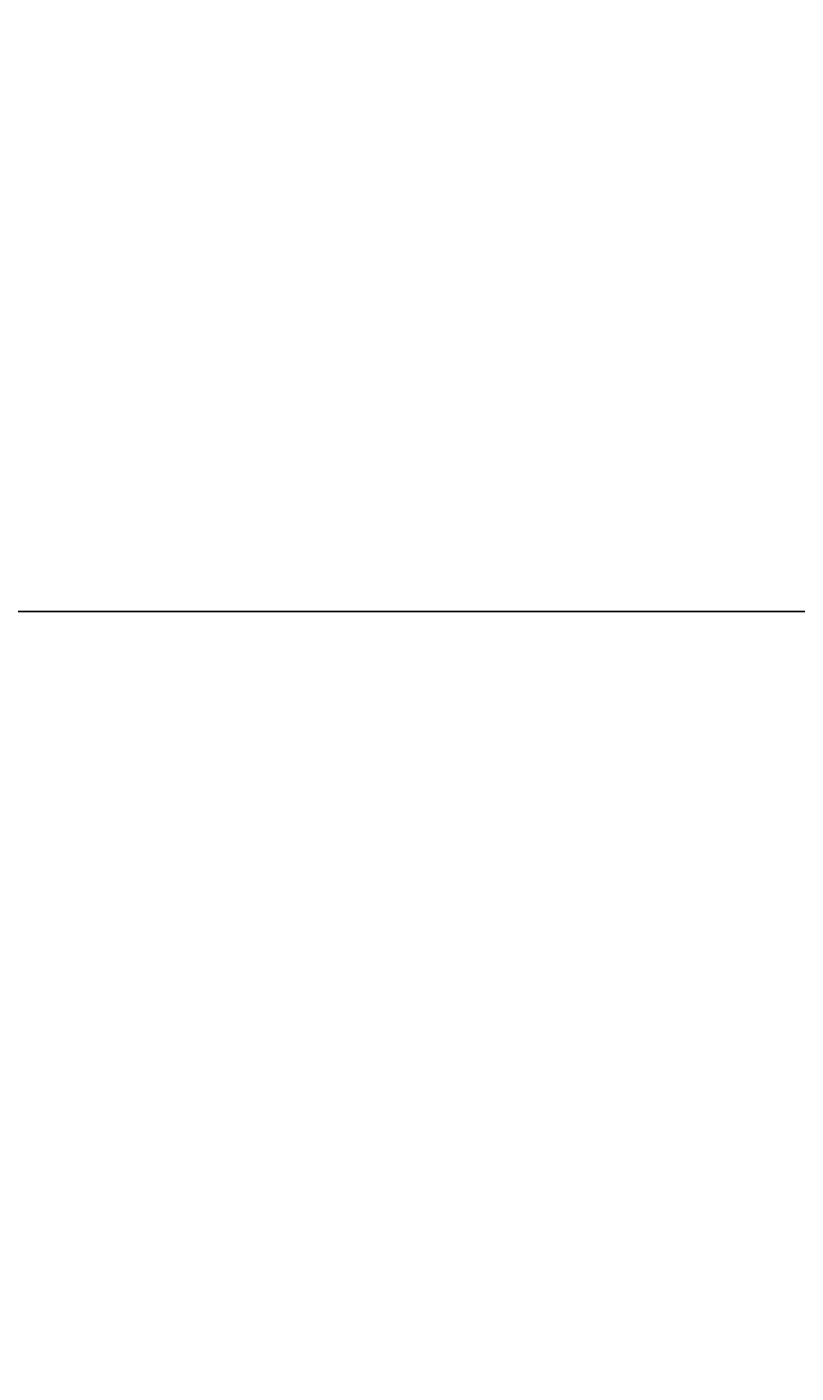
# Model space of a CAD drawing. Units: inches. Extents: x -301 to 715, y -607 to 364.
# Tile 38 of 141: x 101 to 121, y -405 to -370. Entities that reach past the tile are written whole.
import ezdxf

# ---------------------------------------------------------------- set-up
doc = ezdxf.new("R2010")
doc.units = ezdxf.units.IN
doc.header["$MEASUREMENT"] = 0
doc.layers.add('A-ANNO-DIMS', color=2, linetype='Continuous', lineweight=18)
doc.styles.get("Standard").update_dxf_attribs({"font": 'arial.ttf'})
doc.dimstyles.get("Standard").update_dxf_attribs({"dimtxt": 0.18, "dimasz": 0.18, "dimexe": 0.18, "dimexo": 0.0625, "dimgap": 0.09, "dimtad": 0, "dimtih": 1, "dimtoh": 1, "dimdec": 1, "dimzin": 0, "dimdsep": 46, "dimlunit": 4, "dimtxsty": 'Standard', "dimcen": 0.09, "dimclrd": 3, "dimclre": 4, "dimclrt": 6, "dimadec": 0, "dimazin": 0, "dimtfac": 1, "dimtdec": 1, "dimtofl": 0, "dimtmove": 0, "dimatfit": 3, "dimfxl": 1, "dimtfill": 2, "dimtfillclr": 51, "dimtolj": 1, "dimtzin": 0, "dimarcsym": 0})

# ---------------------------------------------------------------- blocks, each defined once
blk = doc.blocks.new('*D176')
at = {"layer": 'A-ANNO-DIMS', "color": 4, "lineweight": -2, "transparency": 16777216}
for p, q in [((148.28, -324.477), (215.605, -324.477)), ((-15.22, -540.477), (215.605, -540.477))]:
    blk.add_line(p, q, dxfattribs=at)
at = {"layer": 'A-ANNO-DIMS', "color": 3, "lineweight": -2, "transparency": 16777216}
for p, q in [((215.425, -324.657), (215.425, -432.296)), ((215.425, -540.297), (215.425, -432.659))]:
    blk.add_line(p, q, dxfattribs=at)
at = {"layer": 'A-ANNO-DIMS', "color": 3, "transparency": 16777216}
for points in [[(215.395, -324.657), (215.455, -324.657), (215.425, -324.477)], [(215.395, -540.297), (215.455, -540.297), (215.425, -540.477)]]:
    blk.add_solid(points, dxfattribs=at)
at = {"layer": 'Defpoints', "color": 0, "transparency": 16777216}
for p in [(148.218, -324.477), (-15.282, -540.477), (215.425, -540.477)]:
    blk.add_point(p, dxfattribs=at)
at = {"layer": 'A-ANNO-DIMS', "color": 6, "transparency": 16777216, "insert": (215.425, -432.477), "char_height": 0.18, "attachment_point": 5, "bg_fill": 1, "box_fill_scale": 1.25, "bg_fill_color": 51, "bg_fill_transparency": 0}
blk.add_mtext('\\A1;18\'-0"', dxfattribs=at)
blk = doc.blocks.new('*D187')
at = {"layer": 'A-ANNO-DIMS', "color": 4, "lineweight": -2, "transparency": 16777216}
for p, q in [((139.674, -385.477), (-266.112, -385.477)), ((143.155, -439.477), (-266.112, -439.477))]:
    blk.add_line(p, q, dxfattribs=at)
at = {"layer": 'A-ANNO-DIMS', "color": 3, "lineweight": -2, "transparency": 16777216}
for p, q in [((-265.932, -385.657), (-265.932, -412.296)), ((-265.932, -439.297), (-265.932, -412.659))]:
    blk.add_line(p, q, dxfattribs=at)
at = {"layer": 'A-ANNO-DIMS', "color": 3, "transparency": 16777216}
for points in [[(-265.962, -385.657), (-265.902, -385.657), (-265.932, -385.477)], [(-265.962, -439.297), (-265.902, -439.297), (-265.932, -439.477)]]:
    blk.add_solid(points, dxfattribs=at)
at = {"layer": 'Defpoints', "color": 0, "transparency": 16777216}
for p in [(-265.932, -385.477), (139.737, -385.477), (143.218, -439.477)]:
    blk.add_point(p, dxfattribs=at)
at = {"layer": 'A-ANNO-DIMS', "color": 6, "transparency": 16777216, "insert": (-265.932, -412.477), "char_height": 0.18, "attachment_point": 5, "bg_fill": 1, "box_fill_scale": 1.25, "bg_fill_color": 51, "bg_fill_transparency": 0}
blk.add_mtext('\\A1;4\'-6"', dxfattribs=at)

msp = doc.modelspace()

# ---------------------------------------------------------------- dimensions: what is measured, and where the dimension line sits
at = {"layer": 'A-ANNO-DIMS'}
for base, p1, p2, picture, middle in [((215.425, -540.477), (148.218, -324.477), (-15.282, -540.477), '*D176', (215.425, -432.477)), ((-265.932, -385.477), (143.218, -439.477), (139.737, -385.477), '*D187', (-265.932, -412.477))]:
    dim = msp.add_linear_dim(base=base, p1=p1, p2=p2, angle=90, dimstyle='Standard', override={"dimdec": 1, "dimlfac": 1, "dimrnd": 0, "dimzin": 1, "dimdsep": 46, "dimlunit": 4, "dimfrac": 2}, dxfattribs=at)
    dim.commit()
    dim.dimension.update_dxf_attribs({"geometry": picture, "text_midpoint": middle})

doc.saveas('drawing.dxf')
